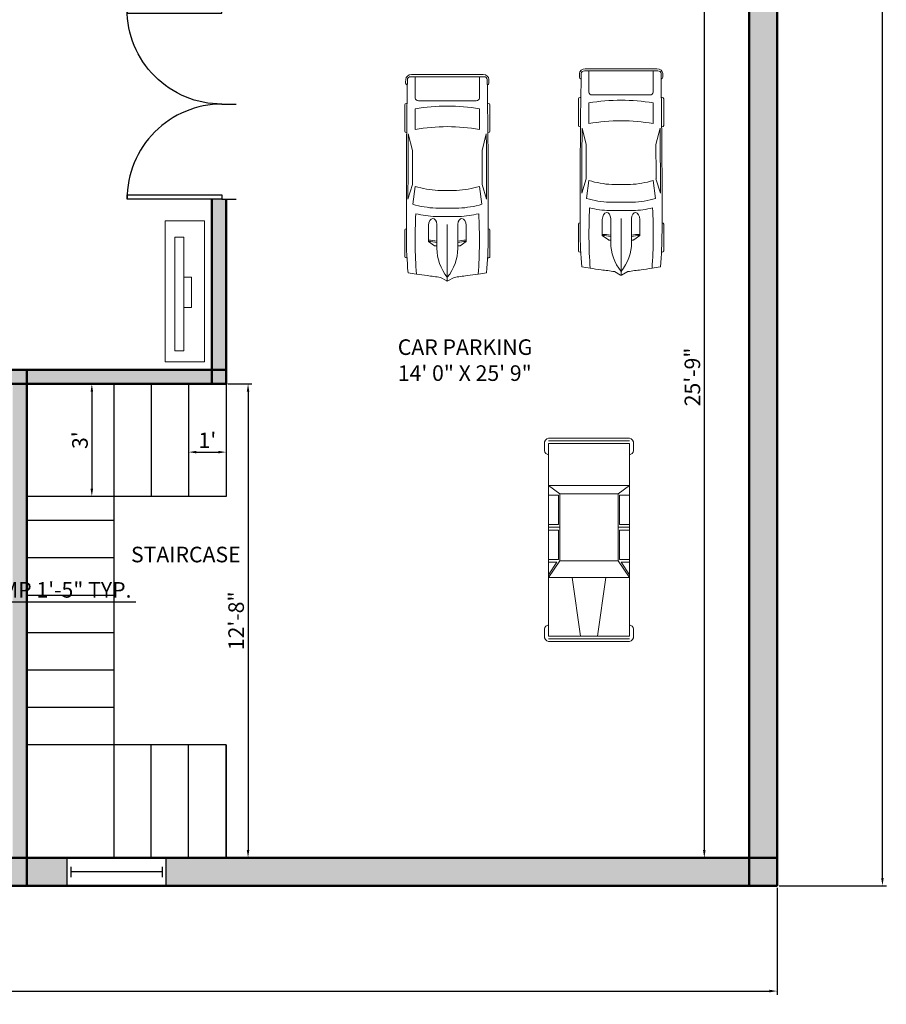
# Model space of a CAD drawing. Units: millimetres. Extents: x 3107 to 3757, y 777 to 1464.
# Tile 3 of 7: x 3479 to 3757, y 824 to 1140. Entities that reach past the tile are written whole.
import ezdxf

# ---------------------------------------------------------------- set-up
doc = ezdxf.new("R2010")
doc.units = ezdxf.units.MM
for name, color, linetype, lineweight in [('A-ANNO-DIMS', 50, 'Continuous', 18), ('A-AREA-IDEN', 160, 'Continuous', 18), ('A-EQPM', 140, 'Continuous', 18), ('A-EQPM-VEHC', 140, 'Continuous', 13), ('A-WALL-PATT', 80, 'Continuous', 13), ('doors', 10, 'Continuous', 25), ('staircase', 190, 'Continuous', 25), ('walls', 80, 'Continuous', 50), ('windows', 30, 'Continuous', 25)]:
    doc.layers.add(name, color=color, linetype=linetype, lineweight=lineweight)
doc.styles.get("Standard").update_dxf_attribs({"font": 'arial.ttf'})
doc.dimstyles.new('ISO-25', dxfattribs={"dimtxt": 5, "dimasz": 2.5, "dimexe": 1.25, "dimexo": 0.625, "dimtad": 1, "dimdec": 0, "dimlunit": 3, "dimtxsty": 'Standard', "dimcen": 2.5, "dimadec": 0, "dimazin": 0, "dimtfac": 1, "dimtdec": 0, "dimtmove": 0, "dimatfit": 3, "dimfxl": 1, "dimarcsym": 0})

# ---------------------------------------------------------------- blocks, each defined once
blk = doc.blocks.new('*U2')
for p, q in [((0, 0), (0, -6)), ((40, 0), (40, -6))]:
    blk.add_line(p, q)
blk.add_lwpolyline([(0, 0), (0, 40), (1.75, 40), (1.75, 0)], close=True)
blk.add_arc((0, 0), 40, 0, 90)
blk = doc.blocks.new('*U5')
for p, q in [((0, 4), (0, 0)), ((36, 4), (36, 0)), ((0, 2), (36, 2))]:
    blk.add_line(p, q)
blk = doc.blocks.new('*U14')
for p, q in [((21.1, 37.41), (21.1, 36.83)), ((46.55, 38.89), (22.35, 38.89)), ((47.8, 37.39), (47.8, 37.41)), ((135.45, 37.07), (135.45, 37.41)), ((136.7, 38.89), (160.9, 38.89)), ((162.15, 37.41), (162.15, 36.77)), ((70.03, 31.54), (86.41, 29.35)), ((87.99, 31.87), (74.76, 35.92)), ((134.31, 35.6), (119.29, 31.78)), ((138.42, 29.35), (157.25, 29.35)), ((186.47, 29.35), (167.01, 29.35)), ((186.47, -33.5), (186.47, 33.5)), ((188.4, -32.76), (188.4, 32.76)), ((164.52, 26.39), (164.52, -26.39)), ((29.77, 9.51), (51.68, 9.51)), ((32.12, 9.51), (32.12, 11.15)), ((32.27, 11.63), (36.13, 17.17)), ((36.13, 17.17), (50.94, 17.17)), ((58.92, -10.77), (58.92, 10.77)), ((66.55, -10.53), (66.55, 10.53)), ((186.47, -10.53), (186.47, 10.53)), ((3.27, 6.13), (0.1, 0.41)), ((82.74, 8.5), (82.74, -8.5)), ((0, 0), (51.68, 0)), ((0.1, -0.41), (3.27, -6.13)), ((29.77, -9.51), (51.68, -9.51)), ((32.12, -9.51), (32.12, -11.15)), ((32.27, -11.63), (36.13, -17.17)), ((36.13, -17.17), (50.94, -17.17)), ((86.41, -29.35), (70.03, -31.54)), ((87.99, -31.87), (74.76, -35.92)), ((134.31, -35.6), (119.29, -31.78)), ((157.25, -29.35), (138.42, -29.35)), ((167.01, -29.35), (186.47, -29.35)), ((21.1, -37.41), (21.1, -36.83)), ((46.55, -38.89), (22.35, -38.89)), ((47.8, -37.39), (47.8, -37.41)), ((135.45, -37.07), (135.45, -37.41)), ((136.7, -38.89), (160.9, -38.89)), ((162.15, -37.41), (162.15, -36.77))]:
    blk.add_line(p, q)
for centre, major_axis, ratio, start_param, end_param in [((41.19, -490.86), (0, 528.23), 0.842304, 0.00281, 0.075598), ((22.35, 37.41), (0, -1.48), 0.842304, 3.141593, 4.712389), ((64.48, -10555.62), (0, 10593.03), 0.842304, -0.013397, 0.002797), ((46.55, 37.41), (0, 1.48), 0.842304, -1.570796, 0), ((136.7, 37.41), (0, -1.48), 0.842304, 3.141593, 4.712389), ((160.9, 37.41), (0, 1.48), 0.842304, -1.570796, 0), ((180.63, 35.84), (0, 2.22), 0.842304, -0.013017, 1.249894), ((64.48, -10556.36), (0, 10595.31), 0.842304, -0.013397, -0.013017), ((183.98, 33.5), (0, -2.96), 0.842304, 1.570796, 3.128196), ((183.98, 32.76), (0, -5.25), 0.842304, 1.570796, 3.128196), ((259.18, -27.52), (0, -305.3), 0.842304, 4.528606, 4.561838), ((266.03, -27.52), (0, 313.31), 0.842304, 1.367076, 1.39176), ((37.47, -593.96), (0, -623.33), 0.842304, 3.096046, 3.200911), ((134.4, 5.39), (0, -89.78), 0.842304, 4.449482, 4.652344), ((135.29, 5.39), (0, 81.77), 0.842304, 1.245306, 1.50788), ((64.48, -10555.62), (0, -10591.55), 0.842304, 3.133765, 3.140441), ((149.6, 2.8), (0, -79.58), 0.842304, 4.372215, 4.640744), ((95.79, -3666.35), (0, -3698.24), 0.842304, 3.134049, 3.144098), ((17.08, 0), (0, 147.02), 0.842304, 4.511394, 4.913384), ((35.91, 0), (0, 147.02), 0.842304, 4.511394, 4.913384), ((167.01, 26.39), (0, 2.96), 0.842304, 0, 1.570796), ((-204.49, 52.4), (0, -250.96), 0.842304, 1.385369, 1.434372), ((29.77, -46.66), (0, 56.17), 0.842304, 0, 0.590319), ((32.75, 11.15), (0, 0.74), 0.842304, 0.879714, 1.570796), ((13.04, 17.01), (0, 27.42), 0.842304, 4.435146, 4.718221), ((14.2, 17.01), (0, 27.42), 0.842304, 4.435146, 4.718221), ((50.79, 13.34), (6.34, -0.36), 0.603834, -1.395552, 1.581315), ((0.62, 0), (0, -0.74), 0.842304, 4.131459, 5.293319), ((-204.49, -52.4), (0, 250.96), 0.842304, -1.434372, -1.385369), ((29.77, 46.66), (0, 56.17), 0.842304, 2.551274, 3.141593), ((149.6, -2.8), (0, -79.58), 0.842304, -1.499151, -1.230623), ((32.75, -11.15), (0, -0.74), 0.842304, 4.712389, 5.403472), ((13.04, -17.01), (0, -27.42), 0.842304, 1.564964, 1.848039), ((14.2, -17.01), (0, -27.42), 0.842304, 1.564964, 1.848039), ((134.4, -5.39), (0, -89.78), 0.842304, -1.510751, -1.307889), ((135.29, -5.39), (0, -81.77), 0.842304, -1.50788, -1.245306), ((259.18, 27.52), (0, 305.3), 0.842304, 1.721348, 1.754579), ((167.01, -26.39), (0, -2.96), 0.842304, 4.712389, 6.283185), ((266.03, 27.52), (0, 313.31), 0.842304, 1.749832, 1.774517), ((37.47, 593.96), (0, -623.33), 0.842304, -0.059319, 0.045547), ((41.19, 490.86), (0, -528.23), 0.842304, -0.075598, -0.00281), ((64.48, 10555.62), (0, -10591.55), 0.842304, 0.001152, 0.007828), ((95.79, 3666.35), (0, -3698.24), 0.842304, -0.002505, 0.007544), ((183.98, -33.5), (0, 2.96), 0.842304, 3.15499, 4.712389), ((183.98, -32.76), (0, -5.25), 0.842304, 0.013397, 1.570796), ((22.35, -37.41), (0, 1.48), 0.842304, 1.570796, 3.141593), ((64.48, 10555.62), (0, 10593.03), 0.842304, 3.138796, 3.15499), ((46.55, -37.41), (0, -1.48), 0.842304, 0, 1.570796), ((136.7, -37.41), (0, -1.48), 0.842304, -1.570796, 0), ((160.9, -37.41), (0, 1.48), 0.842304, 3.141593, 4.712389), ((180.63, -35.84), (0, -2.22), 0.842304, -1.249894, 0.013017), ((64.48, 10556.36), (0, 10595.31), 0.842304, 3.15461, 3.15499)]:
    blk.add_ellipse(centre, major_axis=major_axis, ratio=ratio, start_param=start_param, end_param=end_param)
at = {"extrusion": (0, 0, -1)}
blk.add_ellipse((50.79, -13.34), major_axis=(6.34, 0.36), ratio=0.603834, start_param=-1.395552, end_param=1.581315, dxfattribs=at)
blk = doc.blocks.new('*U15')
for p, q in [((0.1, -0.41), (0.1, 38.35)), ((2.77, -0.41), (2.77, 38.31)), ((5.44, 42.31), (12.12, 42.31)), ((5.44, -0.41), (5.44, 38.24)), ((5.45, 38.31), (16.12, 38.31)), ((16.12, 38.31), (180.34, 38.31)), ((61.52, -0.41), (61.52, 38.31)), ((61.52, 38.31), (77.54, 27.62)), ((64.19, 38.31), (76.2, 30.29)), ((76.2, 30.29), (76.2, 38.31)), ((78.87, 38.31), (78.87, 28.96)), ((106.91, 28.96), (106.91, 38.31)), ((109.58, 27.62), (109.58, 38.31)), ((112.25, 38.31), (112.25, 28.96)), ((140.29, 28.96), (140.29, 38.31)), ((141.62, 27.62), (149.64, 38.31)), ((149.64, -0.41), (149.64, 38.31)), ((189.69, 38.31), (179.01, 38.31)), ((189.69, 42.31), (183.01, 42.31)), ((189.69, -0.41), (189.69, 38.24)), ((192.36, -0.41), (192.36, 38.31)), ((195.03, -0.41), (195.03, 38.35)), ((78.87, 28.96), (106.91, 28.96)), ((112.25, 28.96), (140.29, 28.96)), ((77.54, 27.62), (141.62, 27.62)), ((77.54, -0.41), (77.54, 27.62)), ((141.62, -0.41), (141.62, 27.62)), ((5.44, 7.6), (61.52, 15.61)), ((0.1, -0.42), (0.1, -39.18)), ((2.77, -0.41), (2.77, -39.13)), ((5.44, -0.42), (5.44, -39.07)), ((5.44, -8.42), (61.52, -16.43)), ((61.52, -0.41), (61.52, -39.13)), ((77.54, -0.41), (77.54, -28.45)), ((141.62, -0.41), (141.62, -28.45)), ((149.64, -0.41), (149.64, -39.13)), ((189.69, -0.42), (189.69, -39.07)), ((192.36, -0.41), (192.36, -39.13)), ((195.03, -0.42), (195.03, -39.18)), ((61.52, -39.13), (77.54, -28.45)), ((64.19, -39.13), (76.2, -31.12)), ((76.2, -31.12), (76.2, -39.13)), ((77.54, -28.45), (141.62, -28.45)), ((78.87, -39.13), (78.87, -29.79)), ((78.87, -29.79), (106.91, -29.79)), ((106.91, -29.79), (106.91, -39.13)), ((109.58, -28.45), (109.58, -39.13)), ((112.25, -29.79), (140.29, -29.79)), ((112.25, -39.13), (112.25, -29.79)), ((140.29, -29.79), (140.29, -39.13)), ((141.62, -28.45), (149.64, -39.13)), ((5.44, -43.14), (12.12, -43.14)), ((5.45, -39.13), (16.12, -39.13)), ((16.12, -39.13), (180.34, -39.13)), ((189.69, -39.13), (179.01, -39.13)), ((189.69, -43.14), (183.01, -43.14))]:
    blk.add_line(p, q)
for centre, radius, start, end in [((5.06, 37.26), 5.06, 85.64554, 168.0943), ((11.45, 37.64), 4.72, 8.13011, 81.86996), ((183.68, 37.64), 4.72, 98.13004, 171.8699), ((190.07, 37.26), 5.06, 11.90574, 94.35446), ((5.06, -38.09), 5.06, 191.9057, 274.3545), ((11.45, -38.46), 4.72, 278.13, 351.8699), ((183.68, -38.46), 4.72, 188.1301, 261.87), ((190.07, -38.09), 5.06, 265.6455, 348.0943)]:
    blk.add_arc(centre, radius, start, end)
blk = doc.blocks.new('*D43')
at = {"layer": 'A-ANNO-DIMS', "color": 0, "lineweight": -2, "transparency": 16777216}
for p, q in [((3694.45, 1179.93), (3699.81, 1179.93)), ((3698.56, 1177.43), (3698.56, 873.93)), ((3687.78, 871.43), (3699.81, 871.43))]:
    blk.add_line(p, q, dxfattribs=at)
at = {"layer": 'A-ANNO-DIMS', "color": 0, "transparency": 16777216}
for points in [[(3698.14, 1177.43), (3698.97, 1177.43), (3698.56, 1179.93)], [(3698.14, 873.93), (3698.97, 873.93), (3698.56, 871.43)]]:
    blk.add_solid(points, dxfattribs=at)
at = {"layer": 'Defpoints', "color": 0, "transparency": 16777216}
for p in [(3693.82, 1179.93), (3687.15, 871.43), (3698.56, 871.43)]:
    blk.add_point(p, dxfattribs=at)
at = {"layer": 'A-ANNO-DIMS', "color": 0, "transparency": 16777216, "insert": (3695.38, 1025.68), "char_height": 5, "attachment_point": 5, "rotation": 90}
blk.add_mtext('25\'-9"', dxfattribs=at)
blk = doc.blocks.new('*D44')
at = {"layer": 'A-ANNO-DIMS', "color": 0, "lineweight": -2, "transparency": 16777216}
for p, q in [((3535.47, 1001.57), (3542.47, 1001.57)), ((3544.97, 1001.85), (3544.97, 1000.32)), ((3532.97, 1001.19), (3532.97, 1000.32))]:
    blk.add_line(p, q, dxfattribs=at)
at = {"layer": 'A-ANNO-DIMS', "color": 0, "transparency": 16777216}
for points in [[(3535.47, 1001.99), (3535.47, 1001.16), (3532.97, 1001.57)], [(3542.47, 1001.99), (3542.47, 1001.16), (3544.97, 1001.57)]]:
    blk.add_solid(points, dxfattribs=at)
at = {"layer": 'Defpoints', "color": 0, "transparency": 16777216}
for p in [(3532.97, 1001.82), (3544.97, 1002.47), (3544.97, 1001.57)]:
    blk.add_point(p, dxfattribs=at)
at = {"layer": 'A-ANNO-DIMS', "color": 0, "transparency": 16777216, "insert": (3538.97, 1004.71), "char_height": 5, "attachment_point": 5}
blk.add_mtext("1'", dxfattribs=at)
blk = doc.blocks.new('*D45')
at = {"layer": 'A-ANNO-DIMS', "color": 0, "lineweight": -2, "transparency": 16777216}
for p, q in [((3520.34, 1023.43), (3500.64, 1023.43)), ((3501.89, 1020.93), (3501.89, 989.87)), ((3520.34, 987.37), (3500.64, 987.37))]:
    blk.add_line(p, q, dxfattribs=at)
at = {"layer": 'A-ANNO-DIMS', "color": 0, "transparency": 16777216}
for points in [[(3501.48, 1020.93), (3502.31, 1020.93), (3501.89, 1023.43)], [(3501.48, 989.87), (3502.31, 989.87), (3501.89, 987.37)]]:
    blk.add_solid(points, dxfattribs=at)
at = {"layer": 'Defpoints', "color": 0, "transparency": 16777216}
for p in [(3520.97, 1023.43), (3501.89, 987.37), (3520.97, 987.37)]:
    blk.add_point(p, dxfattribs=at)
at = {"layer": 'A-ANNO-DIMS', "color": 0, "transparency": 16777216, "insert": (3498.72, 1005.4), "char_height": 5, "attachment_point": 5, "rotation": 90}
blk.add_mtext("3'", dxfattribs=at)
blk = doc.blocks.new('*D46')
at = {"layer": 'A-ANNO-DIMS', "color": 0, "lineweight": -2, "transparency": 16777216}
for p, q in [((3545.59, 1023.43), (3553.3, 1023.43)), ((3552.05, 1020.93), (3552.05, 873.93)), ((3545.59, 871.43), (3553.3, 871.43))]:
    blk.add_line(p, q, dxfattribs=at)
at = {"layer": 'A-ANNO-DIMS', "color": 0, "transparency": 16777216}
for points in [[(3551.63, 1020.93), (3552.47, 1020.93), (3552.05, 1023.43)], [(3551.63, 873.93), (3552.47, 873.93), (3552.05, 871.43)]]:
    blk.add_solid(points, dxfattribs=at)
at = {"layer": 'Defpoints', "color": 0, "transparency": 16777216}
for p in [(3544.97, 1023.43), (3544.97, 871.43), (3552.05, 871.43)]:
    blk.add_point(p, dxfattribs=at)
at = {"layer": 'A-ANNO-DIMS', "color": 0, "transparency": 16777216, "insert": (3548.87, 947.43), "char_height": 5, "attachment_point": 5, "rotation": 90}
blk.add_mtext('12\'-8"', dxfattribs=at)
blk = doc.blocks.new('*D63')
at = {"layer": 'A-ANNO-DIMS', "color": 0, "lineweight": -2, "transparency": 16777216}
for p, q in [((3443.96, 955.48), (3443.96, 952.3)), ((3461, 955.48), (3461, 952.3)), ((3446.46, 953.55), (3458.5, 953.55)), ((3461, 953.55), (3515.97, 953.55))]:
    blk.add_line(p, q, dxfattribs=at)
at = {"layer": 'A-ANNO-DIMS', "color": 0, "transparency": 16777216}
for points in [[(3446.46, 953.96), (3446.46, 953.13), (3443.96, 953.55)], [(3458.5, 953.96), (3458.5, 953.13), (3461, 953.55)]]:
    blk.add_solid(points, dxfattribs=at)
at = {"layer": 'Defpoints', "color": 0, "transparency": 16777216}
for p in [(3443.96, 956.1), (3461, 956.1), (3461, 953.55)]:
    blk.add_point(p, dxfattribs=at)
at = {"layer": 'A-ANNO-DIMS', "color": 0, "transparency": 16777216, "insert": (3489.74, 956.72), "char_height": 5, "attachment_point": 5}
blk.add_mtext('LAMP 1\'-5" TYP.', dxfattribs=at)
blk = doc.blocks.new('*D69')
at = {"layer": 'A-ANNO-DIMS', "color": 0, "lineweight": -2, "transparency": 16777216}
for p, q in [((3110.47, 861.8), (3110.47, 827.39)), ((3721.97, 861.8), (3721.97, 827.39)), ((3112.97, 828.64), (3719.47, 828.64))]:
    blk.add_line(p, q, dxfattribs=at)
at = {"layer": 'A-ANNO-DIMS', "color": 0, "transparency": 16777216}
for points in [[(3112.97, 829.06), (3112.97, 828.22), (3110.47, 828.64)], [(3719.47, 829.06), (3719.47, 828.22), (3721.97, 828.64)]]:
    blk.add_solid(points, dxfattribs=at)
at = {"layer": 'Defpoints', "color": 0, "transparency": 16777216}
for p in [(3110.47, 862.43), (3721.97, 862.43), (3721.97, 828.64)]:
    blk.add_point(p, dxfattribs=at)
at = {"layer": 'A-ANNO-DIMS', "color": 0, "transparency": 16777216, "insert": (3416.22, 831.85), "char_height": 5, "attachment_point": 5}
blk.add_mtext('50\'-11 1/2"', dxfattribs=at)
blk = doc.blocks.new('*D70')
at = {"layer": 'A-ANNO-DIMS', "color": 0, "lineweight": -2, "transparency": 16777216}
for p, q in [((3722.59, 1450.43), (3757.01, 1450.43)), ((3755.76, 864.93), (3755.76, 1447.93)), ((3722.59, 862.43), (3757.01, 862.43))]:
    blk.add_line(p, q, dxfattribs=at)
at = {"layer": 'A-ANNO-DIMS', "color": 0, "transparency": 16777216}
for points in [[(3755.34, 1447.93), (3756.17, 1447.93), (3755.76, 1450.43)], [(3755.34, 864.93), (3756.17, 864.93), (3755.76, 862.43)]]:
    blk.add_solid(points, dxfattribs=at)
at = {"layer": 'Defpoints', "color": 0, "transparency": 16777216}
for p in [(3721.97, 1450.43), (3755.76, 1450.43), (3721.97, 862.43)]:
    blk.add_point(p, dxfattribs=at)
at = {"layer": 'A-ANNO-DIMS', "color": 0, "transparency": 16777216, "insert": (3752.58, 1156.43), "char_height": 5, "attachment_point": 5, "rotation": 90}
blk.add_mtext('49\'-0"', dxfattribs=at)

msp = doc.modelspace()

# ---------------------------------------------------------------- hatches: boundary and pattern name
at = {"layer": 'A-WALL-PATT'}
h = msp.add_hatch(color=256, dxfattribs=at)
h.dxf.hatch_style = 1
h.paths.add_polyline_path([(3119.47, 1087.39), (3110.47, 1087.39), (3110.47, 1027.93), (3119.47, 1027.93)])
h.paths.add_polyline_path([(3119.47, 1027.93), (3110.47, 1027.93), (3110.47, 1023.43), (3119.47, 1023.43)])
h.paths.add_polyline_path([(3267.47, 1027.93), (3119.47, 1027.93), (3119.47, 1023.43), (3267.47, 1023.43)])
h.paths.add_polyline_path([(3119.47, 1023.43), (3110.47, 1023.43), (3110.47, 979.44), (3119.47, 979.44)])
h.paths.add_polyline_path([(3299.97, 1179.93), (3295.47, 1179.93), (3295.47, 1027.93), (3299.97, 1027.93)])
h.paths.add_polyline_path([(3295.47, 1027.93), (3271.97, 1027.93), (3271.97, 1023.43), (3295.47, 1023.43)])
h.paths.add_polyline_path([(3271.97, 1027.93), (3267.47, 1027.93), (3267.47, 1023.43), (3271.97, 1023.43)])
h.paths.add_polyline_path([(3299.97, 1027.93), (3295.47, 1027.93), (3295.47, 1023.43), (3299.97, 1023.43)])
h.paths.add_polyline_path([(3299.97, 1184.43), (3295.47, 1184.43), (3295.47, 1179.93), (3299.97, 1179.93)])
h.paths.add_polyline_path([(3295.47, 1184.43), (3288.38, 1184.43), (3288.38, 1182.47), (3288.38, 1179.93), (3295.47, 1179.93)])
h.paths.add_polyline_path([(3352.47, 1179.93), (3347.97, 1179.93), (3347.97, 1027.93), (3352.47, 1027.93)])
h.paths.add_polyline_path([(3352.47, 1184.43), (3347.97, 1184.43), (3347.97, 1179.93), (3352.47, 1179.93)])
h.paths.add_polyline_path([(3464.47, 1184.43), (3352.47, 1184.43), (3352.47, 1179.93), (3464.47, 1179.93)])
h.paths.add_polyline_path([(3468.97, 1288.93), (3464.47, 1288.93), (3464.47, 1184.43), (3468.97, 1184.43)])
h.paths.add_polyline_path([(3468.97, 1184.43), (3464.47, 1184.43), (3464.47, 1179.93), (3468.97, 1179.93)])
h.paths.add_polyline_path([(3195.97, 1248.43), (3191.47, 1248.43), (3191.47, 1184.43), (3195.97, 1184.43)])
h.paths.add_polyline_path([(3195.97, 1184.43), (3191.47, 1184.43), (3191.47, 1179.93), (3195.97, 1179.93)])
h.paths.add_polyline_path([(3191.47, 1184.43), (3183.28, 1184.43), (3183.28, 1181.58), (3183.28, 1179.93), (3191.47, 1179.93)])
h.paths.add_polyline_path([(3243.97, 1184.43), (3195.97, 1184.43), (3195.97, 1179.93), (3243.97, 1179.93)])
h.paths.add_polyline_path([(3257.91, 1182.47), (3257.91, 1184.43), (3248.47, 1184.43), (3248.47, 1179.93), (3258.02, 1179.93, -0.020891)])
h.paths.add_polyline_path([(3248.47, 1184.43), (3243.97, 1184.43), (3243.97, 1179.93), (3248.47, 1179.93)])
h.paths.add_polyline_path([(3248.47, 1189.24), (3247.51, 1189.24), (3243.97, 1189.24), (3243.97, 1184.43), (3248.47, 1184.43)])
h.paths.add_polyline_path([(3166.87, 1184.43), (3119.47, 1184.43), (3119.47, 1179.93), (3166.63, 1179.93), (3166.63, 1181.58, -0.042981)])
h.paths.add_polyline_path([(3119.47, 1184.43), (3110.47, 1184.43), (3110.47, 1179.93), (3119.47, 1179.93)])
h.paths.add_polyline_path([(3119.47, 1248.43), (3110.47, 1248.43), (3110.47, 1184.43), (3119.47, 1184.43)])
h.paths.add_polyline_path([(3119.47, 1179.93), (3110.47, 1179.93), (3110.47, 1140.65), (3119.47, 1140.65)])
h.paths.add_polyline_path([(3119.47, 1288.93), (3110.47, 1288.93), (3110.47, 1252.93), (3119.47, 1252.93)])
h.paths.add_polyline_path([(3119.47, 1252.93), (3110.47, 1252.93), (3110.47, 1248.43), (3119.47, 1248.43)])
h.paths.add_polyline_path([(3191.47, 1252.93), (3119.47, 1252.93), (3119.47, 1248.43), (3191.47, 1248.43)])
h.paths.add_polyline_path([(3195.97, 1288.93), (3191.47, 1288.93), (3191.47, 1252.93), (3195.97, 1252.93)])
h.paths.add_polyline_path([(3195.97, 1252.93), (3191.47, 1252.93), (3191.47, 1248.43), (3195.97, 1248.43)])
h.paths.add_polyline_path([(3248.47, 1293.43), (3243.97, 1293.43), (3243.97, 1288.93), (3248.47, 1288.93)])
h.paths.add_polyline_path([(3243.97, 1293.43), (3195.97, 1293.43), (3195.97, 1288.93), (3243.97, 1288.93)])
h.paths.add_polyline_path([(3303.47, 1293.43), (3248.47, 1293.43), (3248.47, 1288.93), (3303.47, 1288.93)])
h.paths.add_polyline_path([(3248.47, 1288.93), (3243.97, 1288.93), (3243.97, 1205.51, -0.053712), (3247.51, 1205.89), (3248.47, 1205.89)])
h.paths.add_polyline_path([(3191.47, 1293.43), (3119.47, 1293.43), (3119.47, 1288.93), (3191.47, 1288.93)])
h.paths.add_polyline_path([(3119.47, 1293.43), (3110.47, 1293.43), (3110.47, 1288.93), (3119.47, 1288.93)])
h.paths.add_polyline_path([(3119.47, 1322.96, -0.065064), (3111.64, 1321.93), (3110.47, 1321.93), (3110.47, 1293.43), (3119.47, 1293.43)])
h.paths.add_polyline_path([(3195.97, 1293.43), (3191.47, 1293.43), (3191.47, 1288.93), (3195.97, 1288.93)])
h.paths.add_polyline_path([(3119.47, 1450.43), (3110.47, 1450.43), (3110.47, 1441.43), (3119.47, 1441.43)])
h.paths.add_polyline_path([(3119.47, 1441.43), (3110.47, 1441.43), (3110.47, 1352.4), (3111.64, 1352.4), (3119.47, 1352.4)])
h.paths.add_polyline_path([(3176.58, 1450.43), (3119.47, 1450.43), (3119.47, 1441.43), (3176.58, 1441.43)])
h.paths.add_polyline_path([(3323.19, 1450.43), (3307.97, 1450.43), (3307.97, 1441.43), (3323.19, 1441.43)])
h.paths.add_polyline_path([(3307.97, 1450.43), (3303.47, 1450.43), (3303.47, 1441.43), (3307.97, 1441.43)])
h.paths.add_polyline_path([(3303.47, 1450.43), (3229.4, 1450.43), (3229.4, 1441.43), (3303.47, 1441.43)])
h.paths.add_polyline_path([(3307.97, 1441.43), (3303.47, 1441.43), (3303.47, 1363.43), (3307.97, 1363.43)])
h.paths.add_polyline_path([(3307.97, 1363.43), (3303.47, 1363.43), (3303.47, 1358.93), (3307.97, 1358.93)])
h.paths.add_polyline_path([(3307.97, 1358.93), (3303.47, 1358.93), (3303.47, 1342.3), (3305.5, 1342.3, -0.037178), (3307.97, 1342.12)])
h.paths.add_polyline_path([(3379.97, 1363.43), (3307.97, 1363.43), (3307.97, 1358.93), (3379.97, 1358.93)])
h.paths.add_polyline_path([(3384.47, 1393.61), (3383.04, 1393.61), (3379.97, 1393.61), (3379.97, 1363.43), (3384.47, 1363.43)])
h.paths.add_polyline_path([(3384.47, 1363.43), (3379.97, 1363.43), (3379.97, 1358.93), (3384.47, 1358.93)])
h.paths.add_polyline_path([(3384.47, 1358.93), (3379.97, 1358.93), (3379.97, 1293.43), (3384.47, 1293.43)])
h.paths.add_polyline_path([(3384.47, 1441.43), (3379.97, 1441.43), (3379.97, 1409.98, -0.046389), (3383.04, 1410.27), (3384.47, 1410.27)])
h.paths.add_polyline_path([(3384.47, 1450.43), (3379.97, 1450.43), (3379.97, 1441.43), (3384.47, 1441.43)])
h.paths.add_polyline_path([(3379.97, 1450.43), (3357.18, 1450.43), (3357.18, 1441.43), (3379.97, 1441.43)])
h.paths.add_polyline_path([(3432.79, 1450.43), (3384.47, 1450.43), (3384.47, 1441.43), (3432.79, 1441.43)])
h.paths.add_polyline_path([(3540.47, 1450.43), (3484.18, 1450.43), (3484.18, 1441.43), (3540.47, 1441.43)])
h.paths.add_polyline_path([(3544.97, 1450.43), (3540.47, 1450.43), (3540.47, 1441.43), (3544.97, 1441.43)])
h.paths.add_polyline_path([(3544.97, 1441.43), (3540.47, 1441.43), (3540.47, 1293.43), (3544.97, 1293.43)])
h.paths.add_polyline_path([(3590.83, 1450.43), (3544.97, 1450.43), (3544.97, 1441.43), (3590.83, 1441.43)])
h.paths.add_polyline_path([(3712.97, 1450.43), (3645.62, 1450.43), (3645.62, 1441.43), (3712.97, 1441.43)])
h.paths.add_polyline_path([(3721.97, 1441.43), (3712.97, 1441.43), (3712.97, 1288.93), (3712.97, 1184.43), (3721.97, 1184.43), (3721.97, 1288.93)])
h.paths.add_polyline_path([(3721.97, 1450.43), (3712.97, 1450.43), (3712.97, 1441.43), (3721.97, 1441.43)])
h.paths.add_polyline_path([(3712.97, 1184.43), (3658.24, 1184.43), (3658.24, 1183.15), (3658.24, 1179.93), (3712.97, 1179.93)])
h.paths.add_polyline_path([(3721.97, 1184.43), (3712.97, 1184.43), (3712.97, 1179.93), (3721.97, 1179.93)])
h.paths.add_polyline_path([(3597.32, 1183.15), (3597.32, 1184.43), (3544.97, 1184.43), (3544.97, 1179.93), (3597.32, 1179.93)])
h.paths.add_polyline_path([(3544.97, 1184.43), (3540.47, 1184.43), (3540.47, 1179.93), (3544.97, 1179.93)])
h.paths.add_polyline_path([(3544.97, 1179.93), (3540.47, 1179.93), (3540.47, 1143.69), (3543.65, 1143.69), (3544.97, 1143.69)])
h.paths.add_polyline_path([(3721.97, 1179.93), (3712.97, 1179.93), (3712.97, 1006.22), (3712.97, 871.43), (3721.97, 871.43), (3721.97, 1006.22)])
h.paths.add_polyline_path([(3468.97, 1293.43), (3464.47, 1293.43), (3464.47, 1288.93), (3468.97, 1288.93)])
h.paths.add_polyline_path([(3540.47, 1293.43), (3468.97, 1293.43), (3468.97, 1288.93), (3540.47, 1288.93)])
h.paths.add_polyline_path([(3544.97, 1293.43), (3540.47, 1293.43), (3540.47, 1288.93), (3544.97, 1288.93)])
h.paths.add_polyline_path([(3464.47, 1293.43), (3417.83, 1293.43, -0.015057), (3417.88, 1291.6), (3417.88, 1288.93), (3464.47, 1288.93)])
h.paths.add_polyline_path([(3379.97, 1293.43), (3307.97, 1293.43), (3307.97, 1288.93), (3379.97, 1288.93)])
h.paths.add_polyline_path([(3307.97, 1325.65), (3305.5, 1325.65), (3303.47, 1325.65), (3303.47, 1293.43), (3307.97, 1293.43)])
h.paths.add_polyline_path([(3307.97, 1293.43), (3303.47, 1293.43), (3303.47, 1288.93), (3307.97, 1288.93)])
h.paths.add_polyline_path([(3384.47, 1293.43), (3379.97, 1293.43), (3379.97, 1288.93), (3384.47, 1288.93)])
h.paths.add_polyline_path([(3387.42, 1291.6), (3387.42, 1293.43), (3384.47, 1293.43), (3384.47, 1288.93), (3387.42, 1288.93)])
h.paths.add_polyline_path([(3119.47, 927.28), (3110.47, 927.28), (3110.47, 871.43), (3119.47, 871.43)])
h.paths.add_polyline_path([(3119.47, 871.43), (3110.47, 871.43), (3110.47, 862.43), (3119.47, 862.43)])
h.paths.add_polyline_path([(3267.47, 871.43), (3119.47, 871.43), (3119.47, 862.43), (3267.47, 862.43)])
h.paths.add_polyline_path([(3271.97, 971.43), (3267.47, 971.43), (3267.47, 871.43), (3271.97, 871.43)])
h.paths.add_polyline_path([(3271.97, 871.43), (3267.47, 871.43), (3267.47, 862.43), (3271.97, 862.43)])
h.paths.add_polyline_path([(3287.13, 871.43), (3271.97, 871.43), (3271.97, 862.43), (3287.13, 862.43)])
h.paths.add_polyline_path([(3347.97, 871.43), (3318.96, 871.43), (3318.96, 862.43), (3347.97, 862.43)])
h.paths.add_polyline_path([(3352.47, 971.43), (3347.97, 971.43), (3347.97, 871.43), (3352.47, 871.43)])
h.paths.add_polyline_path([(3352.47, 871.43), (3347.97, 871.43), (3347.97, 862.43), (3352.47, 862.43)])
h.paths.add_polyline_path([(3375.96, 871.43), (3352.47, 871.43), (3352.47, 862.43), (3375.96, 862.43)])
h.paths.add_polyline_path([(3352.47, 975.93), (3347.97, 975.93), (3347.97, 971.43), (3352.47, 971.43)])
h.paths.add_polyline_path([(3352.47, 986.27, -0.01722), (3350.37, 986.2), (3347.97, 986.2), (3347.97, 975.93), (3352.47, 975.93)])
h.paths.add_polyline_path([(3347.97, 975.93), (3292.38, 975.93), (3292.38, 973.47, -0.030785), (3292.25, 971.43), (3347.97, 971.43)])
h.paths.add_polyline_path([(3271.97, 985.98), (3269.95, 985.98), (3267.47, 985.98), (3267.47, 975.93), (3271.97, 975.93)])
h.paths.add_polyline_path([(3271.97, 975.93), (3267.47, 975.93), (3267.47, 971.43), (3271.97, 971.43)])
h.paths.add_polyline_path([(3275.72, 975.93), (3271.97, 975.93), (3271.97, 971.43), (3275.72, 971.43), (3275.72, 973.47)])
h.paths.add_polyline_path([(3271.97, 1023.43), (3267.47, 1023.43), (3267.47, 1016.34, -0.020418), (3269.95, 1016.44), (3271.97, 1016.44)])
h.paths.add_polyline_path([(3352.47, 1023.43), (3347.97, 1023.43), (3347.97, 1016.67), (3350.37, 1016.67), (3352.47, 1016.67)])
h.paths.add_polyline_path([(3352.47, 1027.93), (3347.97, 1027.93), (3347.97, 1023.43), (3352.47, 1023.43)])
h.paths.add_polyline_path([(3476.47, 1027.93), (3352.47, 1027.93), (3352.47, 1023.43), (3476.47, 1023.43)])
h.paths.add_polyline_path([(3540.47, 1027.93), (3480.97, 1027.93), (3480.97, 1023.43), (3540.47, 1023.43)])
h.paths.add_polyline_path([(3480.97, 1027.93), (3476.47, 1027.93), (3476.47, 1023.43), (3480.97, 1023.43)])
h.paths.add_polyline_path([(3480.97, 1023.43), (3476.47, 1023.43), (3476.47, 871.43), (3480.97, 871.43)])
h.paths.add_polyline_path([(3476.47, 871.43), (3429.88, 871.43), (3429.88, 862.43), (3476.47, 862.43)])
h.paths.add_polyline_path([(3480.97, 871.43), (3476.47, 871.43), (3476.47, 862.43), (3480.97, 862.43)])
h.paths.add_polyline_path([(3493.81, 871.43), (3480.97, 871.43), (3480.97, 862.43), (3493.81, 862.43)])
h.paths.add_polyline_path([(3712.97, 871.43), (3525.61, 871.43), (3525.61, 862.43), (3712.97, 862.43)])
h.paths.add_polyline_path([(3721.97, 871.43), (3712.97, 871.43), (3712.97, 862.43), (3721.97, 862.43)])
h = msp.add_hatch(color=256, dxfattribs=at)
h.dxf.hatch_style = 1
h.paths.add_polyline_path([(3544.97, 1082.76), (3543.65, 1082.76), (3540.47, 1082.76), (3540.47, 1027.93), (3544.97, 1027.93)])
h.paths.add_polyline_path([(3544.97, 1027.93), (3540.47, 1027.93), (3540.47, 1023.43), (3544.97, 1023.43)])

# ---------------------------------------------------------------- linework, layer by layer
at = {"layer": 'A-EQPM'}
for points in [[(3538.09, 1075.82), (3525.48, 1075.82), (3525.48, 1030.54), (3538.09, 1030.54)], [(3528.51, 1070.57), (3531.43, 1070.57), (3531.43, 1034.04), (3528.51, 1034.04)], [(3531.43, 1057.74), (3533.86, 1057.74), (3533.86, 1047.96), (3531.43, 1047.96)]]:
    msp.add_lwpolyline(points, close=True, dxfattribs=at)
at = {"layer": 'staircase'}
for p, q in [((3508.97, 1023.43), (3508.97, 871.43)), ((3520.97, 1023.43), (3520.97, 987.37)), ((3532.97, 1023.43), (3532.97, 987.37)), ((3544.97, 1023.43), (3544.97, 987.37)), ((3544.97, 987.37), (3480.97, 987.37)), ((3508.97, 979.61), (3480.97, 979.61)), ((3508.97, 967.61), (3480.97, 967.61)), ((3508.97, 955.61), (3480.97, 955.61)), ((3508.97, 943.61), (3480.97, 943.61)), ((3508.97, 931.61), (3480.97, 931.61)), ((3508.97, 919.61), (3480.97, 919.61)), ((3544.97, 907.61), (3480.97, 907.61)), ((3520.97, 871.43), (3520.97, 907.61)), ((3532.97, 871.43), (3532.97, 907.61)), ((3544.97, 871.43), (3544.97, 907.61)), ((3544.97, 907.61), (3544.97, 871.43))]:
    msp.add_line(p, q, dxfattribs=at)
at = {"layer": 'walls'}
for p, q in [((3712.97, 1288.93), (3712.97, 1006.22)), ((3721.97, 1288.93), (3721.97, 1006.22)), ((3540.47, 1082.76), (3540.47, 1023.43)), ((3544.97, 1082.76), (3544.97, 1023.43)), ((3347.97, 1027.93), (3544.97, 1027.93)), ((3480.97, 1027.93), (3480.97, 862.43)), ((3347.97, 1023.43), (3544.97, 1023.43)), ((3712.97, 1006.22), (3712.97, 862.43)), ((3721.97, 1006.22), (3721.97, 862.43)), ((3110.47, 871.43), (3721.97, 871.43)), ((3110.47, 862.43), (3721.97, 862.43))]:
    msp.add_line(p, q, dxfattribs=at)
at = {"layer": 'windows'}
for p, q in [((3493.81, 871.43), (3493.81, 862.43)), ((3525.61, 871.43), (3525.61, 862.43))]:
    msp.add_line(p, q, dxfattribs=at)

# ---------------------------------------------------------------- block references
at = {"layer": 'A-EQPM-VEHC'}
for name, p, xscale, yscale, zscale, rotation in [('*U14', (3616.03, 1056.45), 0.3515837203701919, 0.3515837203701919, 0.3515837203701919, 90), ('*U14', (3671.84, 1058.33), 0.3515837203701919, 0.3515837203701919, 0.3515837203701919, 90), ('*U15', (3661.39, 940.72), 0.335124271855346, 0.335124271855346, 0.335124271855346, 89.99999999999996)]:
    msp.add_blockref(name, p, dxfattribs=dict(at, xscale=xscale, yscale=yscale, zscale=zscale, rotation=rotation))
at = {"layer": 'doors', "yscale": 0.7615706373352984, "zscale": 0.7615706373352984}
for p, xscale, rotation in [((3543.65, 1143.69), -0.7615706373352984, 90.00000000000007), ((3543.65, 1082.76), 0.7615706373352984, 89.99999999999991)]:
    msp.add_blockref('*U2', p, dxfattribs=dict(at, xscale=xscale, rotation=rotation))
at = {"layer": 'windows', "xscale": 0.8150463067894532, "yscale": 0.8150463067894532, "zscale": 0.8150463067894532, "rotation": 180}
msp.add_blockref('*U5', (3524.57, 868.48), dxfattribs=at)

# ---------------------------------------------------------------- texts
at = {"layer": 'A-AREA-IDEN', "char_height": 5, "attachment_point": 1}
for s, width, insert in [('CAR PARKING \\P14\' 0" X 25\' 9"', 49.166, (3600.14, 1037.75)), ('STAIRCASE', 37.5856, (3514.46, 971.21))]:
    msp.add_mtext_dynamic_manual_height_columns(s, width=width, gutter_width=12.5, heights=[0], dxfattribs=dict(at, insert=insert))

# ---------------------------------------------------------------- dimensions: what is measured, and where the dimension line sits
at = {"layer": 'A-ANNO-DIMS'}
for base, p1, p2, override, picture, middle in [((3755.76, 1450.43), (3721.97, 862.43), (3721.97, 1450.43), {"dimdec": 1, "dimlfac": 1, "dimrnd": 0, "dimzin": 1, "dimdsep": 46, "dimlunit": 4, "dimfrac": 2}, '*D70', (3752.58, 1156.43)), ((3698.55806305, 871.42857409), (3693.82046366, 1179.92857409), (3687.15261964, 871.42857409), {"dimclrd": 0, "dimclre": 0, "dimclrt": 0}, '*D43', (3695.38019811, 1025.67857409)), ((3501.89, 987.37), (3520.97, 1023.43), (3520.97, 987.37), {"dimclrd": 0, "dimclre": 0, "dimclrt": 0}, '*D45', (3498.72, 1005.4)), ((3552.05, 871.43), (3544.97, 1023.43), (3544.97, 871.43), {"dimclrd": 0, "dimclre": 0, "dimclrt": 0}, '*D46', (3548.87, 947.43))]:
    dim = msp.add_linear_dim(base=base, p1=p1, p2=p2, angle=90, dimstyle='ISO-25', override=override, dxfattribs=at)
    dim.commit()
    dim.dimension.update_dxf_attribs({"geometry": picture, "text_midpoint": middle})
for base, p1, p2, override, picture, middle in [((3544.97, 1001.57), (3532.97, 1001.82), (3544.97, 1002.47), {"dimclrd": 0, "dimclre": 0, "dimclrt": 0}, '*D44', (3538.97, 1004.71)), ((3721.97, 828.64), (3110.47, 862.43), (3721.97, 862.43), {"dimdec": 1, "dimlfac": 1, "dimrnd": 0, "dimzin": 1, "dimdsep": 46, "dimlunit": 4, "dimfrac": 2}, '*D69', (3416.22, 831.85))]:
    dim = msp.add_linear_dim(base=base, p1=p1, p2=p2, dimstyle='ISO-25', override=override, dxfattribs=at)
    dim.commit()
    dim.dimension.update_dxf_attribs({"geometry": picture, "text_midpoint": middle})
dim = msp.add_linear_dim(base=(3461, 953.55), p1=(3443.96, 956.1), p2=(3461, 956.1), text='LAMP <> TYP.', dimstyle='ISO-25', override={"dimdec": 1, "dimlfac": 1, "dimrnd": 0, "dimzin": 1, "dimdsep": 46, "dimlunit": 4, "dimfrac": 2}, dxfattribs=at)
dim.commit()
dim.dimension.update_dxf_attribs({"geometry": '*D63', "text_midpoint": (3489.74, 956.72)})

doc.saveas('drawing.dxf')
